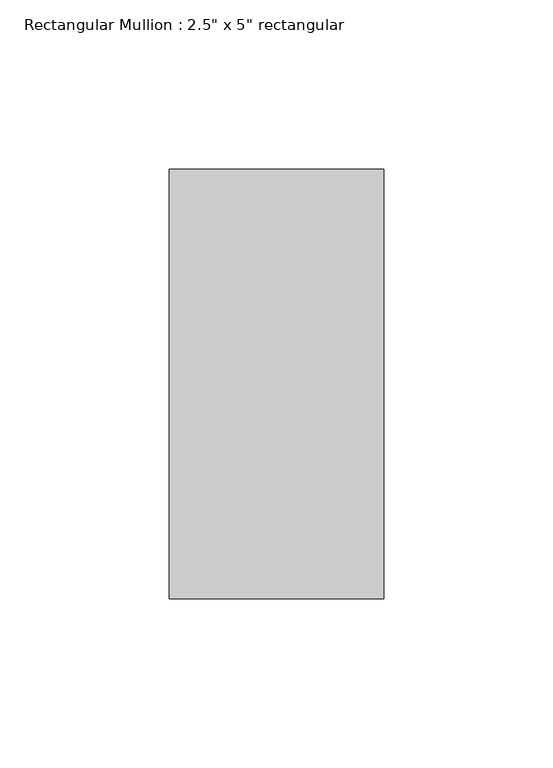
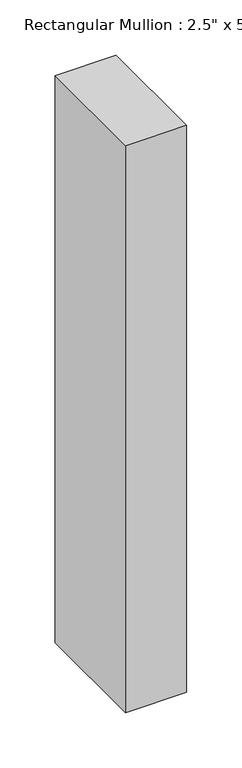
"""IFC4 building model written with IfcOpenShell, lengths in millimetres: member geometry."""

from ifc_helpers import new_model, si_unit, frame, origin, place, context, project, spatial, polyline, outline, extrude, source, transform, mapped, element, save


def member_8c482a5e(model_context):
    return source(origin(), model_context, "Body", "SweptSolid", [
        extrude(outline(polyline([(0.0, 63.5), (0.0, -63.5), (-63.5, -63.5), (-63.5, 63.5), (0.0, 63.5)])), frame((0.0, 0.0, -623.7034682), z_axis=(0.0, 0.0, 1.0), x_axis=(1.0, 0.0, 0.0)), (0.0, 0.0, 1.0), 623.7034682),
    ])


if __name__ == "__main__":
    model = new_model("IFC4")
    model_context = context("Model", 3, world=origin())
    ifc_project = project(units=[si_unit("LENGTHUNIT", "METRE", prefix="MILLI")], contexts=[model_context])
    site = spatial("IfcSite", under=ifc_project)
    building = spatial("IfcBuilding", under=site)
    placement = place(None, origin())
    member_shape = member_8c482a5e(model_context)
    element("IfcMember", 1, ObjectType="Rectangular Mullion : 2.5\" x 5\" rectangular", at=placement, inside=building, context=model_context, shape_type="MappedRepresentation", body=[
        mapped(member_shape, transform((0.0, 0.0, 0.0), x_axis=(1.0, 0.0, 0.0), y_axis=(0.0, 1.0, 0.0), z_axis=(0.0, 0.0, 1.0))),
    ])
    save(model, "model.ifc")

# Revit data of these elements
# Type "Rectangular Mullion : 2.5\" x 5\" rectangular"
#   built-in parameter 1007304 = 0.416667 (stored number, unit not read)
#   built-in parameter 1007301 = 0.104167 (stored number, unit not read)
#   built-in parameter 1007300 = 0.104167 (stored number, unit not read)
# Element 1 (IfcMember, "Rectangular Mullion : 2.5\" x 5\" rectangular")
#   Materials on its faces: "BLACK COLOUR"
# Materials
#   "BLACK COLOUR": class "Generic", colour RGB 120 120 120, transparency 0, Cost = 0
